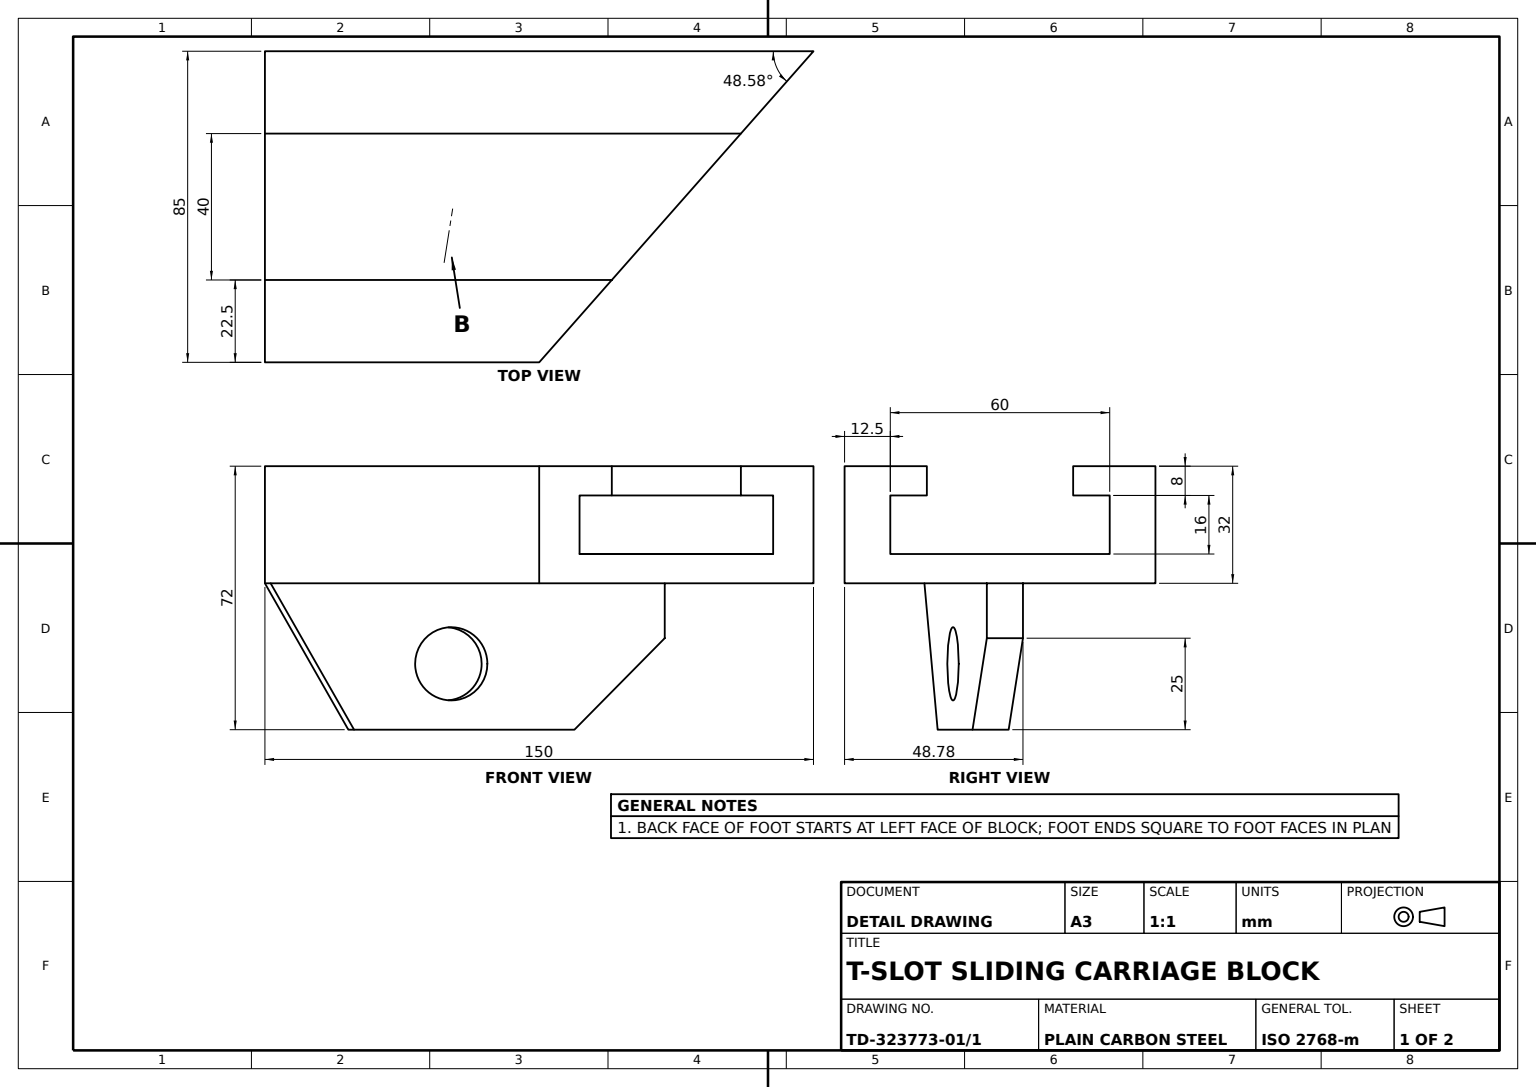
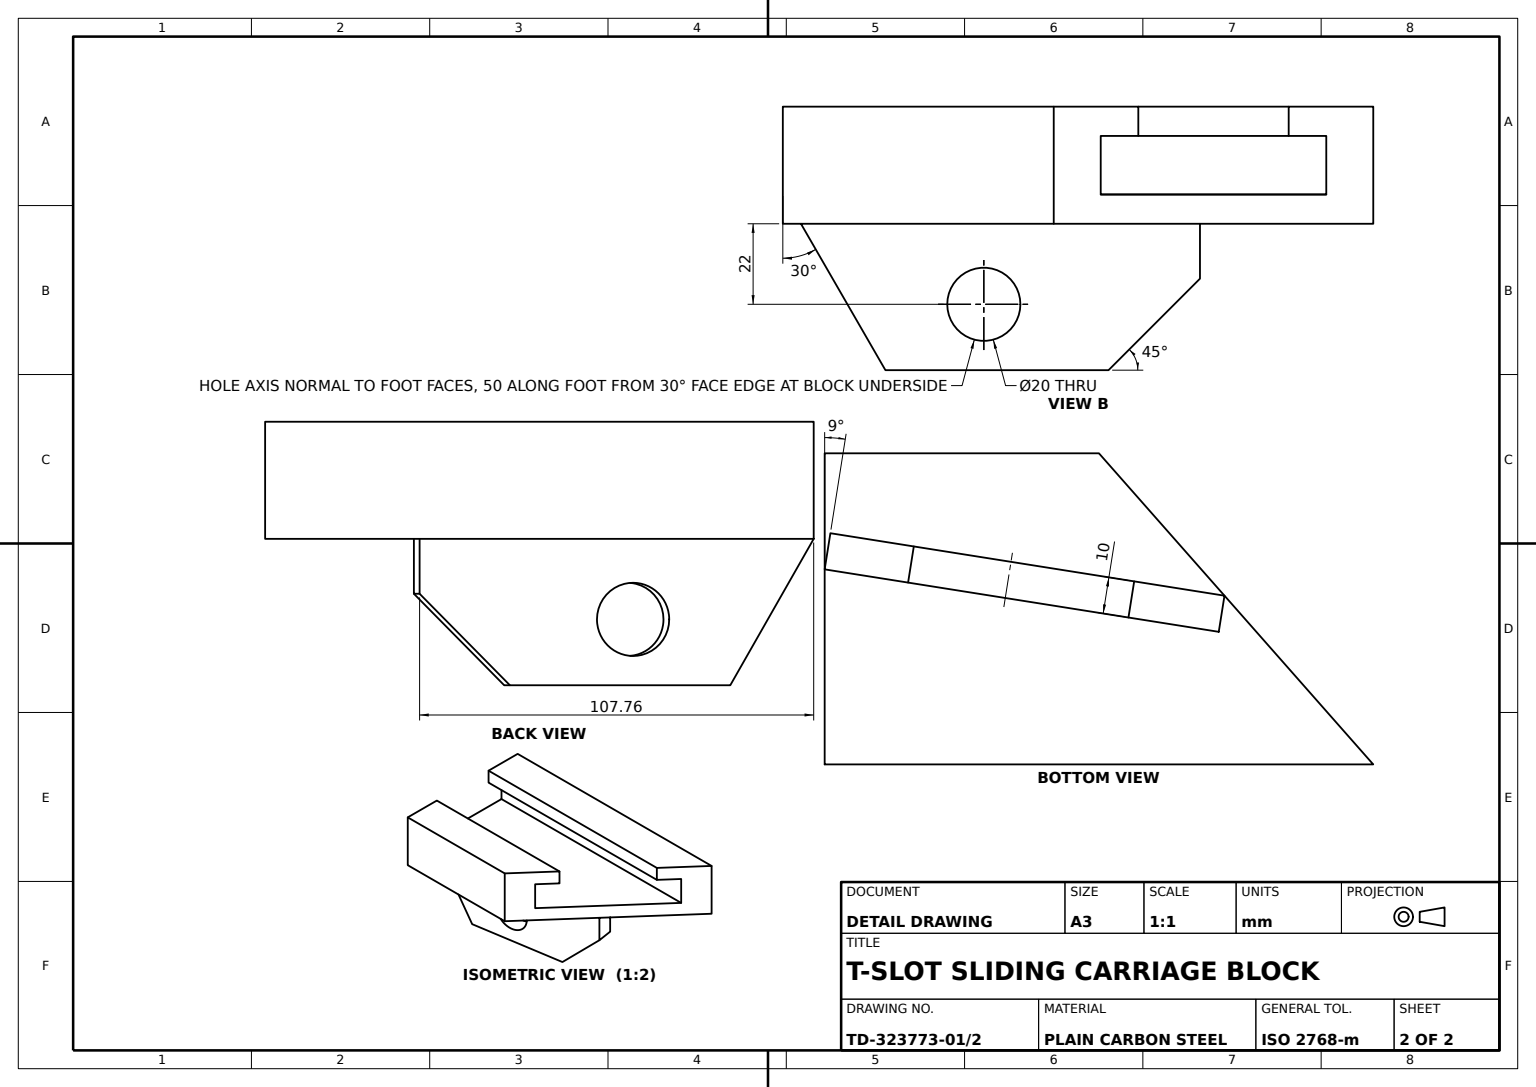
SolidWorks part; units mm, degrees
material "Plain Carbon Steel"
ref_plane "Front Plane" through (0, 0, 0) normal (0, 0, 1) x (1, 0, 0)
ref_plane "Top Plane" through (0, 0, 0) normal (0, 1, 0) x (1, 0, 0)
ref_plane "Right Plane" through (0, 0, 0) normal (1, 0, 0) x (0, 0, -1)
sketch "Base Block Sketch" plane through (0, 0, 0) normal (0, 1, 0) x (1, 0, 0)
  line L1 (-75, 42.5) -> (75, 42.5)
  line L2 (-75, 42.5) -> (-75, -42.5)
  line L3 (-75, -42.5) -> (0, -42.5)
  line L5 (-75, 42.5) -> (75, -42.5) construction
  line L6 (-75, -42.5) -> (75, 42.5) construction
  line L8 (0, -42.5) -> (75, 42.5)
  point P0 (0, 0)
  dimension "D1" = 85
  dimension "D2" = 150
  dimension "D3" = 75
extrude "Base Block 150x85x32" add sketch "Base Block Sketch" along normal blind 32
sketch "T-Slot Sketch" plane through (-75, 0, 0) normal (-1, 0, 0) x (0, 0, 1)
  line L0 (-20, 32) -> (-20, 24)
  line L1 (-30, 8) -> (30, 8)
  line L2 (-30, 8) -> (-30, 24)
  line L3 (-30, 24) -> (-20, 24)
  line L4 (30, 8) -> (30, 24)
  line L5 (-30, 8) -> (30, 24) construction
  line L6 (-30, 24) -> (30, 8) construction
  line L7 (-42.5, 32) -> (42.5, 32) construction
  line L8 (20, 32) -> (20, 24)
  line L9 (20, 24) -> (30, 24)
  line L10 (0, 0) -> (0, 36.7863) construction
  line L15 (-42.5, 0) -> (42.5, 0)
  line L16 (42.5, 0) -> (42.5, 32)
  line L17 (42.5, 32) -> (-42.5, 32)
  line L18 (-42.5, 32) -> (-42.5, 0)
  line L21 (20, 32) -> (-20, 32)
  point P0 (0, 16)
  dimension "D1" = 60
  dimension "D2" = 16
  dimension "D3" = 40
  dimension "D4" = 20
  dimension "D6" = 16
  dimension "D5" = 0
extrude "T-Slot Cut" cut sketch "T-Slot Sketch" against normal through all both and the other way through all
sketch "Tapered Foot Sketch" plane through (0, 0, 0) normal (0, -1, 0) x (1, 0, 0)
  line L0 (-75, 10.7906) -> (-73.4357, 20.6675)
  line L1 (-75, 10.7906) -> (32.759, -6.2767)
  line L2 (-73.4357, 20.6675) -> (34.3234, 3.6002)
  line L3 (32.759, -6.2767) -> (34.3234, 3.6002)
  line L4 (-75, 42.5) -> (0, 42.5) construction
  line L5 (-75, -42.5) -> (-75, 42.5) construction
  line L6 (0, 42.5) -> (75, -42.5) construction
  dimension "D1" = 9
  dimension "D2" = 10
  dimension "D3" = 107.759
extrude "Tapered Foot Boss" add sketch "Tapered Foot Sketch" along normal blind 40
sketch "Foot Relief Sketch" plane through (1.3962, 0, 8.8153) normal (0.1564, 0, 0.9877) x (0.9877, 0, -0.1564)
  line L0 (-75.7647, 0) -> (-52.6706, -40)
  line L1 (33.3376, -40) -> (-75.7647, -40) construction
  line L2 (33.3376, 0) -> (33.3376, -15)
  line L3 (33.3376, -40) -> (33.3376, 0) construction
  line L4 (33.3376, -15) -> (8.3376, -40)
  line L5 (-75.7647, -40) -> (-75.7647, 0) construction
  line L6 (-80.7251, 0) -> (-6.6485, 0) construction
  line L7 (-52.6706, -40) -> (-75.7647, -40)
  line L8 (-75.7647, -40) -> (-75.7647, 0)
  line L9 (8.3376, -40) -> (33.3376, -40)
  line L10 (33.3376, -40) -> (33.3376, -15)
  circle A0 centre (-25.7647, -22) radius 10
  line M4 (-75.7647, 0) -> (-75.7647, -40)
  line M5 (-75.7647, -40) -> (33.3376, -40)
  line M6 (33.3376, -40) -> (33.3376, 0)
  dimension "D2" = 20
  dimension "D1" = 30
  dimension "D3" = 50
  dimension "D4" = 22
  dimension "D5" = 25
  dimension "D6" = 45
  dimension "D7" = 40
extrude "Foot Relief Cut" cut sketch "Foot Relief Sketch" against normal through all both and the other way through all contours L4 M6 M5 | A0 | L0 M4 M5
